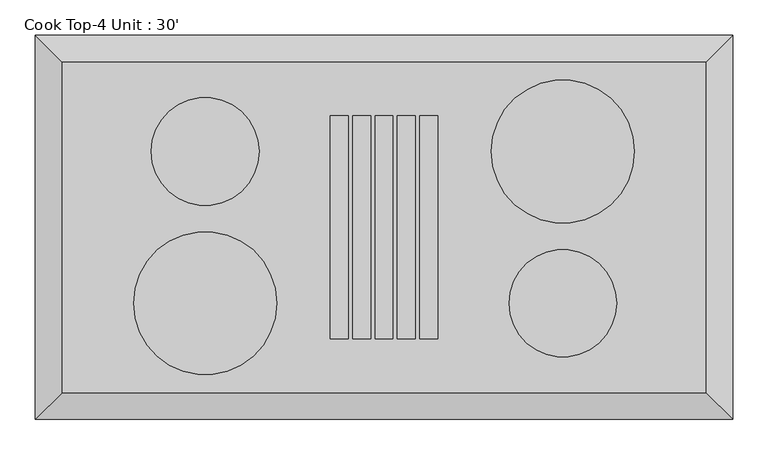
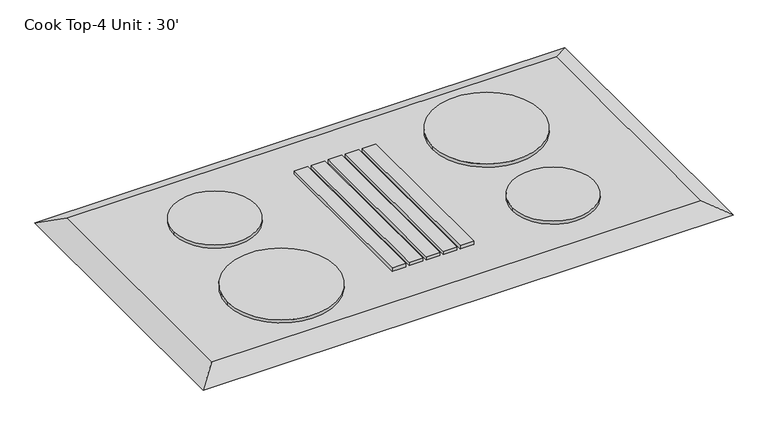
"""IFC4 building model written with IfcOpenShell, lengths in millimetres: proxy geometry, Cook Top-4 Unit : 30'."""

from ifc_helpers import new_model, si_unit, point, frame, frame_2d, origin, place, context, project, spatial, polyline, circle_curve, trimmed, segment, composite_curve, outline, extrude, faceted_brep, source, transform, mapped, element, save


def cook_top_4_unit_30_51a8ed57(model_context):
    return source(origin(), model_context, "Body", "SolidModel", [
        extrude(outline(composite_curve([segment(trimmed(circle_curve(frame_2d((-254.0, 107.7019531)), 76.5869489), [point((-177.4130511, 107.7019531))], [point((-330.5869489, 107.7019531))], False, "CARTESIAN"), True, "CONTINUOUS"), segment(trimmed(circle_curve(frame_2d((-254.0, 107.7019531)), 76.5869489), [point((-330.5869489, 107.7019531))], [point((-177.4130511, 107.7019531))], False, "CARTESIAN"), True, "CONTINUOUS")], self_intersect=False)), frame((0.0, 0.0, 806.45), z_axis=(0.0, 0.0, 1.0), x_axis=(1.0, 0.0, 0.0)), (0.0, 0.0, 1.0), 6.35),
        extrude(outline(composite_curve([segment(trimmed(circle_curve(frame_2d((254.0, 107.7019531)), 101.6), [point((355.6, 107.7019531))], [point((152.4, 107.7019531))], False, "CARTESIAN"), True, "CONTINUOUS"), segment(trimmed(circle_curve(frame_2d((254.0, 107.7019531)), 101.6), [point((152.4, 107.7019531))], [point((355.6, 107.7019531))], False, "CARTESIAN"), True, "CONTINUOUS")], self_intersect=False)), frame((0.0, 0.0, 806.45), z_axis=(0.0, 0.0, 1.0), x_axis=(1.0, 0.0, 0.0)), (0.0, 0.0, 1.0), 6.35),
        extrude(outline(composite_curve([segment(trimmed(circle_curve(frame_2d((254.0, -107.7019531)), 76.2), [point((330.2, -107.7019531))], [point((177.8, -107.7019531))], False, "CARTESIAN"), True, "CONTINUOUS"), segment(trimmed(circle_curve(frame_2d((254.0, -107.7019531)), 76.2), [point((177.8, -107.7019531))], [point((330.2, -107.7019531))], False, "CARTESIAN"), True, "CONTINUOUS")], self_intersect=False)), frame((0.0, 0.0, 806.45), z_axis=(0.0, 0.0, 1.0), x_axis=(1.0, 0.0, 0.0)), (0.0, 0.0, 1.0), 6.35),
        extrude(outline(polyline([(-50.8, 158.5019531), (-50.8, -158.5019531), (-76.2, -158.5019531), (-76.2, 158.5019531), (-50.8, 158.5019531)])), frame((0.0, 0.0, 806.45), z_axis=(0.0, 0.0, 1.0), x_axis=(1.0, 0.0, 0.0)), (0.0, 0.0, 1.0), 6.35),
        extrude(outline(polyline([(-19.05, 158.5019531), (-19.05, -158.5019531), (-44.45, -158.5019531), (-44.45, 158.5019531), (-19.05, 158.5019531)])), frame((0.0, 0.0, 806.45), z_axis=(0.0, 0.0, 1.0), x_axis=(1.0, 0.0, 0.0)), (0.0, 0.0, 1.0), 6.35),
        extrude(outline(polyline([(12.7, 158.5019531), (12.7, -158.5019531), (-12.7, -158.5019531), (-12.7, 158.5019531), (12.7, 158.5019531)])), frame((0.0, 0.0, 806.45), z_axis=(0.0, 0.0, 1.0), x_axis=(1.0, 0.0, 0.0)), (0.0, 0.0, 1.0), 6.35),
        extrude(outline(polyline([(44.45, 158.5019531), (44.45, -158.5019531), (19.05, -158.5019531), (19.05, 158.5019531), (44.45, 158.5019531)])), frame((0.0, 0.0, 806.45), z_axis=(0.0, 0.0, 1.0), x_axis=(1.0, 0.0, 0.0)), (0.0, 0.0, 1.0), 6.35),
        extrude(outline(polyline([(76.2, 158.5019531), (76.2, -158.5019531), (50.8, -158.5019531), (50.8, 158.5019531), (76.2, 158.5019531)])), frame((0.0, 0.0, 806.45), z_axis=(0.0, 0.0, 1.0), x_axis=(1.0, 0.0, 0.0)), (0.0, 0.0, 1.0), 6.35),
        faceted_brep([(457.2, 234.7019531, 806.45), (-457.2, 234.7019531, 806.45), (-457.2, -234.7019531, 806.45), (457.2, -234.7019531, 806.45), (495.3, 272.8019531, 787.4), (495.3, -272.8019531, 787.4), (-495.3, -272.8019531, 787.4), (-495.3, 272.8019531, 787.4)], [[[0, 1, 2, 3]], [[4, 5, 6, 7]], [[4, 7, 1, 0]], [[7, 6, 2, 1]], [[6, 5, 3, 2]], [[5, 4, 0, 3]]]),
        extrude(outline(composite_curve([segment(trimmed(circle_curve(frame_2d((-254.0, -107.7019531)), 101.6), [point((-152.4, -107.7019531))], [point((-355.6, -107.7019531))], False, "CARTESIAN"), True, "CONTINUOUS"), segment(trimmed(circle_curve(frame_2d((-254.0, -107.7019531)), 101.6), [point((-355.6, -107.7019531))], [point((-152.4, -107.7019531))], False, "CARTESIAN"), True, "CONTINUOUS")], self_intersect=False)), frame((0.0, 0.0, 806.45), z_axis=(0.0, 0.0, 1.0), x_axis=(1.0, 0.0, 0.0)), (0.0, 0.0, 1.0), 6.35),
    ])


if __name__ == "__main__":
    model = new_model("IFC4")
    model_context = context("Model", 3, world=origin())
    ifc_project = project(units=[si_unit("LENGTHUNIT", "METRE", prefix="MILLI")], contexts=[model_context])
    site = spatial("IfcSite", under=ifc_project)
    building = spatial("IfcBuilding", under=site)
    placement = place(None, origin())
    cook_top_4_unit_30_shape = cook_top_4_unit_30_51a8ed57(model_context)
    element("IfcBuildingElementProxy", 1, Name="Cook Top-4 Unit : 30'", ObjectType="Cook Top-4 Unit : 30'", at=placement, inside=building, context=model_context, shape_type="MappedRepresentation", body=[
        mapped(cook_top_4_unit_30_shape, transform((0.0, 0.0, 0.0), x_axis=(1.0, 0.0, 0.0), y_axis=(0.0, 1.0, 0.0), z_axis=(0.0, 0.0, 1.0))),
    ])
    save(model, "model.ifc")

# Revit data of these elements
# Type "Cook Top-4 Unit : 30'"
#   Assembly Code = "E1090400"
#   Depth = 1' - 6 123/256"
#   Width = 3' - 0"
#   Burner Material = Steel, Chrome Plated
#   Cooktop Material = Steel, Polished
#   Default Elevation = 0
# Element 1 (IfcBuildingElementProxy, "Cook Top-4 Unit : 30'")
#   Materials on its faces: "Steel, Chrome Plated", "Steel, Polished"
# Materials
#   "Steel, Chrome Plated": class "Metal", colour RGB 17 17 17, transparency 0, Description = "Chromiuim plated steel", Cost = 0
#   "Steel, Polished": class "Metal", colour RGB 192 192 192, transparency 0, Description = "Polished steel", Cost = 0
